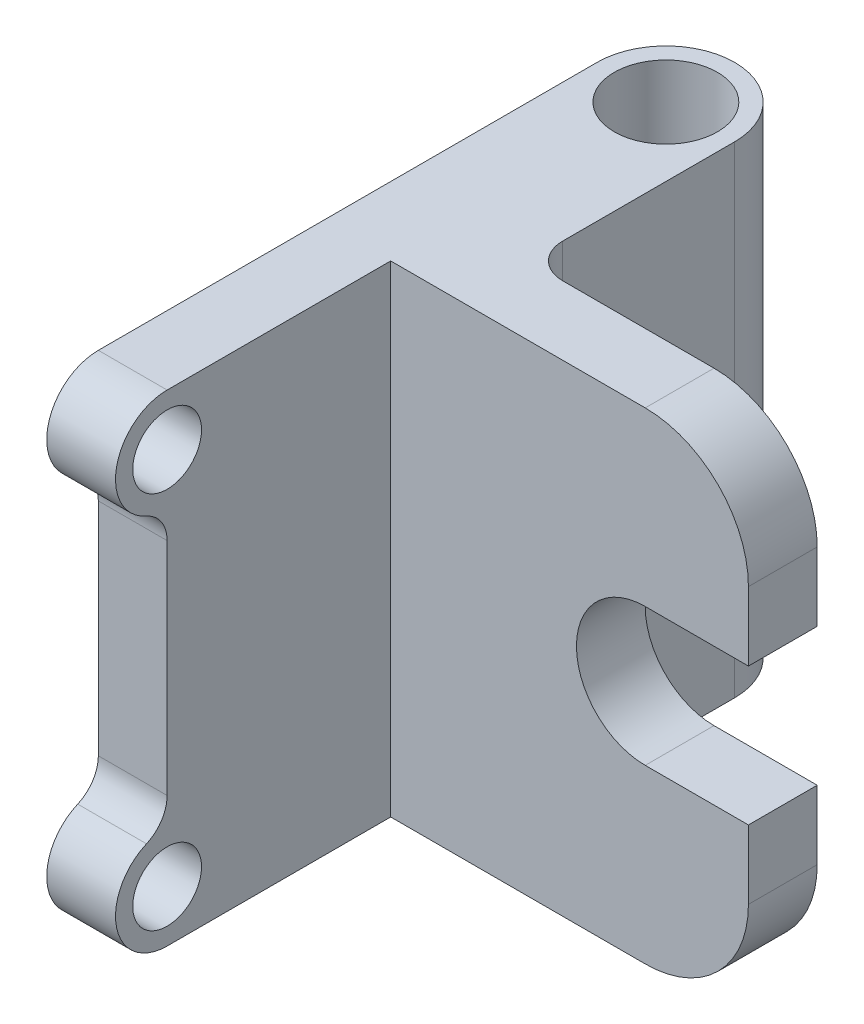
ISO-10303-21;
HEADER;
FILE_DESCRIPTION(('STEP AP214'),'2;1');
FILE_NAME('part.step','',(''),(''),'','','');
FILE_SCHEMA(('AUTOMOTIVE_DESIGN { 1 0 10303 214 1 1 1 1 }'));
ENDSEC;
DATA;
#1=APPLICATION_CONTEXT('core data for automotive mechanical design processes');
#2=APPLICATION_PROTOCOL_DEFINITION('international standard','automotive_design',2000,#1);
#3=PRODUCT_CONTEXT('',#1,'mechanical');
#4=PRODUCT('Part','Part','',(#3));
#5=PRODUCT_RELATED_PRODUCT_CATEGORY('part','',(#4));
#6=PRODUCT_DEFINITION_FORMATION('','',#4);
#7=PRODUCT_DEFINITION_CONTEXT('part definition',#1,'design');
#8=PRODUCT_DEFINITION('design','',#6,#7);
#9=PRODUCT_DEFINITION_SHAPE('','',#8);
#10=(LENGTH_UNIT() NAMED_UNIT(*) SI_UNIT(.MILLI.,.METRE.));
#11=(NAMED_UNIT(*) PLANE_ANGLE_UNIT() SI_UNIT($,.RADIAN.));
#12=(NAMED_UNIT(*) SI_UNIT($,.STERADIAN.) SOLID_ANGLE_UNIT());
#13=UNCERTAINTY_MEASURE_WITH_UNIT(LENGTH_MEASURE(1.E-05),#10,'distance_accuracy_value','');
#14=(GEOMETRIC_REPRESENTATION_CONTEXT(3) GLOBAL_UNCERTAINTY_ASSIGNED_CONTEXT((#13)) GLOBAL_UNIT_ASSIGNED_CONTEXT((#10,
#11,#12)) REPRESENTATION_CONTEXT('',''));
#15=CARTESIAN_POINT('',(0.,0.,0.));
#16=DIRECTION('',(0.,0.,1.));
#17=DIRECTION('',(1.,0.,0.));
#18=AXIS2_PLACEMENT_3D('',#15,#16,#17);
#19=CARTESIAN_POINT('',(47.,15.,0.));
#20=DIRECTION('',(0.,0.,-1.));
#21=DIRECTION('',(-1.,0.,0.));
#22=AXIS2_PLACEMENT_3D('',#19,#20,#21);
#23=PLANE('',#22);
#24=DIRECTION('',(0.,1.,0.));
#25=VECTOR('',#24,1.);
#26=CARTESIAN_POINT('',(25.,0.,0.));
#27=LINE('',#26,#25);
#28=CARTESIAN_POINT('',(25.,0.,0.));
#29=VERTEX_POINT('',#28);
#30=CARTESIAN_POINT('',(25.,70.,0.));
#31=VERTEX_POINT('',#30);
#32=EDGE_CURVE('E69',#29,#31,#27,.T.);
#33=ORIENTED_EDGE('',*,*,#32,.T.);
#34=DIRECTION('',(-1.,0.,0.));
#35=VECTOR('',#34,1.);
#36=CARTESIAN_POINT('',(46.9999999999999,70.,0.));
#37=LINE('',#36,#35);
#38=CARTESIAN_POINT('',(46.9999999999999,70.,0.));
#39=VERTEX_POINT('',#38);
#40=EDGE_CURVE('E270',#39,#31,#37,.T.);
#41=ORIENTED_EDGE('',*,*,#40,.F.);
#42=CARTESIAN_POINT('',(47.,55.,0.));
#43=DIRECTION('',(0.,0.,1.));
#44=DIRECTION('',(1.,0.,0.));
#45=AXIS2_PLACEMENT_3D('',#42,#43,#44);
#46=CIRCLE('',#45,15.);
#47=CARTESIAN_POINT('',(62.,54.9999999999999,0.));
#48=VERTEX_POINT('',#47);
#49=EDGE_CURVE('E296',#48,#39,#46,.T.);
#50=ORIENTED_EDGE('',*,*,#49,.F.);
#51=DIRECTION('',(0.,1.,0.));
#52=VECTOR('',#51,1.);
#53=CARTESIAN_POINT('',(62.,45.,0.));
#54=LINE('',#53,#52);
#55=CARTESIAN_POINT('',(62.,45.,0.));
#56=VERTEX_POINT('',#55);
#57=EDGE_CURVE('E298',#56,#48,#54,.T.);
#58=ORIENTED_EDGE('',*,*,#57,.F.);
#59=DIRECTION('',(1.,0.,0.));
#60=VECTOR('',#59,1.);
#61=CARTESIAN_POINT('',(62.,45.,0.));
#62=LINE('',#61,#60);
#63=CARTESIAN_POINT('',(47.,45.,0.));
#64=VERTEX_POINT('',#63);
#65=EDGE_CURVE('E295',#64,#56,#62,.T.);
#66=ORIENTED_EDGE('',*,*,#65,.F.);
#67=CARTESIAN_POINT('',(47.,35.,0.));
#68=DIRECTION('',(0.,0.,-1.));
#69=DIRECTION('',(1.,0.,0.));
#70=AXIS2_PLACEMENT_3D('',#67,#68,#69);
#71=CIRCLE('',#70,10.);
#72=CARTESIAN_POINT('',(47.,25.,0.));
#73=VERTEX_POINT('',#72);
#74=EDGE_CURVE('E292',#73,#64,#71,.T.);
#75=ORIENTED_EDGE('',*,*,#74,.F.);
#76=DIRECTION('',(-1.,0.,0.));
#77=VECTOR('',#76,1.);
#78=CARTESIAN_POINT('',(47.,25.,0.));
#79=LINE('',#78,#77);
#80=CARTESIAN_POINT('',(62.,25.,0.));
#81=VERTEX_POINT('',#80);
#82=EDGE_CURVE('E287',#81,#73,#79,.T.);
#83=ORIENTED_EDGE('',*,*,#82,.F.);
#84=DIRECTION('',(0.,1.,0.));
#85=VECTOR('',#84,1.);
#86=CARTESIAN_POINT('',(62.,15.0000000000001,0.));
#87=LINE('',#86,#85);
#88=CARTESIAN_POINT('',(62.,15.0000000000001,0.));
#89=VERTEX_POINT('',#88);
#90=EDGE_CURVE('E290',#89,#81,#87,.T.);
#91=ORIENTED_EDGE('',*,*,#90,.F.);
#92=CARTESIAN_POINT('',(47.,15.,0.));
#93=DIRECTION('',(0.,0.,1.));
#94=DIRECTION('',(-1.,0.,0.));
#95=AXIS2_PLACEMENT_3D('',#92,#93,#94);
#96=CIRCLE('',#95,15.);
#97=CARTESIAN_POINT('',(46.9999999999999,0.,0.));
#98=VERTEX_POINT('',#97);
#99=EDGE_CURVE('E289',#98,#89,#96,.T.);
#100=ORIENTED_EDGE('',*,*,#99,.F.);
#101=DIRECTION('',(1.,0.,0.));
#102=VECTOR('',#101,1.);
#103=CARTESIAN_POINT('',(0.,0.,0.));
#104=LINE('',#103,#102);
#105=EDGE_CURVE('E61',#29,#98,#104,.T.);
#106=ORIENTED_EDGE('',*,*,#105,.F.);
#107=EDGE_LOOP('',(#33,#41,#50,#58,#66,#75,#83,#91,#100,#106));
#108=FACE_BOUND('',#107,.T.);
#109=ADVANCED_FACE('F50',(#108),#23,.T.);
#110=CARTESIAN_POINT('',(10.,70.,42.5));
#111=DIRECTION('',(0.,0.,1.));
#112=DIRECTION('',(1.,0.,0.));
#113=AXIS2_PLACEMENT_3D('',#110,#111,#112);
#114=PLANE('',#113);
#115=DIRECTION('',(0.,1.,0.));
#116=VECTOR('',#115,1.);
#117=CARTESIAN_POINT('',(0.,70.,42.5));
#118=LINE('',#117,#116);
#119=CARTESIAN_POINT('',(0.,18.9564392373896,42.5));
#120=VERTEX_POINT('',#119);
#121=CARTESIAN_POINT('',(0.,51.0435607626104,42.5));
#122=VERTEX_POINT('',#121);
#123=EDGE_CURVE('E250',#120,#122,#118,.T.);
#124=ORIENTED_EDGE('',*,*,#123,.F.);
#125=DIRECTION('',(1.,0.,0.));
#126=VECTOR('',#125,1.);
#127=CARTESIAN_POINT('',(0.,18.9564392373896,42.5));
#128=LINE('',#127,#126);
#129=CARTESIAN_POINT('',(10.,18.9564392373896,42.5));
#130=VERTEX_POINT('',#129);
#131=EDGE_CURVE('E230',#120,#130,#128,.T.);
#132=ORIENTED_EDGE('',*,*,#131,.T.);
#133=DIRECTION('',(0.,1.,0.));
#134=VECTOR('',#133,1.);
#135=CARTESIAN_POINT('',(10.,70.,42.5));
#136=LINE('',#135,#134);
#137=CARTESIAN_POINT('',(10.,51.0435607626104,42.5));
#138=VERTEX_POINT('',#137);
#139=EDGE_CURVE('E253',#130,#138,#136,.T.);
#140=ORIENTED_EDGE('',*,*,#139,.T.);
#141=DIRECTION('',(1.,0.,0.));
#142=VECTOR('',#141,1.);
#143=CARTESIAN_POINT('',(0.,51.0435607626104,42.5));
#144=LINE('',#143,#142);
#145=EDGE_CURVE('E239',#122,#138,#144,.T.);
#146=ORIENTED_EDGE('',*,*,#145,.F.);
#147=EDGE_LOOP('',(#124,#132,#140,#146));
#148=FACE_BOUND('',#147,.T.);
#149=ADVANCED_FACE('F360',(#148),#114,.T.);
#150=CARTESIAN_POINT('',(0.,70.,10.));
#151=DIRECTION('',(1.,0.,0.));
#152=DIRECTION('',(0.,0.,-1.));
#153=AXIS2_PLACEMENT_3D('',#150,#151,#152);
#154=PLANE('',#153);
#155=CARTESIAN_POINT('',(0.,62.5,42.5));
#156=DIRECTION('',(1.,0.,0.));
#157=DIRECTION('',(0.,0.,-1.));
#158=AXIS2_PLACEMENT_3D('',#155,#156,#157);
#159=CIRCLE('',#158,5.);
#160=CARTESIAN_POINT('',(0.,62.5,37.5));
#161=VERTEX_POINT('',#160);
#162=EDGE_CURVE('E209',#161,#161,#159,.T.);
#163=ORIENTED_EDGE('',*,*,#162,.T.);
#164=EDGE_LOOP('',(#163));
#165=FACE_BOUND('',#164,.T.);
#166=CARTESIAN_POINT('',(0.,7.5,42.5));
#167=DIRECTION('',(1.,0.,0.));
#168=DIRECTION('',(0.,0.,-1.));
#169=AXIS2_PLACEMENT_3D('',#166,#167,#168);
#170=CIRCLE('',#169,5.);
#171=CARTESIAN_POINT('',(0.,7.5,37.5));
#172=VERTEX_POINT('',#171);
#173=EDGE_CURVE('E205',#172,#172,#170,.T.);
#174=ORIENTED_EDGE('',*,*,#173,.T.);
#175=EDGE_LOOP('',(#174));
#176=FACE_BOUND('',#175,.T.);
#177=DIRECTION('',(0.,0.,-1.));
#178=VECTOR('',#177,1.);
#179=CARTESIAN_POINT('',(0.,70.,10.));
#180=LINE('',#179,#178);
#181=CARTESIAN_POINT('',(0.,70.,42.5));
#182=VERTEX_POINT('',#181);
#183=CARTESIAN_POINT('',(0.,70.,-30.));
#184=VERTEX_POINT('',#183);
#185=EDGE_CURVE('E198',#182,#184,#180,.T.);
#186=ORIENTED_EDGE('',*,*,#185,.T.);
#187=DIRECTION('',(0.,-1.,0.));
#188=VECTOR('',#187,1.);
#189=CARTESIAN_POINT('',(0.,70.,-30.));
#190=LINE('',#189,#188);
#191=CARTESIAN_POINT('',(0.,0.,-30.));
#192=VERTEX_POINT('',#191);
#193=EDGE_CURVE('E177',#184,#192,#190,.T.);
#194=ORIENTED_EDGE('',*,*,#193,.T.);
#195=DIRECTION('',(0.,0.,-1.));
#196=VECTOR('',#195,1.);
#197=CARTESIAN_POINT('',(0.,0.,10.));
#198=LINE('',#197,#196);
#199=CARTESIAN_POINT('',(0.,0.,42.5));
#200=VERTEX_POINT('',#199);
#201=EDGE_CURVE('E11',#200,#192,#198,.T.);
#202=ORIENTED_EDGE('',*,*,#201,.F.);
#203=CARTESIAN_POINT('',(0.,7.5,42.5));
#204=DIRECTION('',(1.,0.,0.));
#205=DIRECTION('',(0.,0.,-1.));
#206=AXIS2_PLACEMENT_3D('',#203,#204,#205);
#207=CIRCLE('',#206,7.50000000000001);
#208=CARTESIAN_POINT('',(0.,14.3738635424338,45.5));
#209=VERTEX_POINT('',#208);
#210=EDGE_CURVE('E224',#209,#200,#207,.T.);
#211=ORIENTED_EDGE('',*,*,#210,.F.);
#212=CARTESIAN_POINT('',(0.,18.9564392373896,47.5));
#213=DIRECTION('',(1.,0.,0.));
#214=DIRECTION('',(0.,0.,-1.));
#215=AXIS2_PLACEMENT_3D('',#212,#213,#214);
#216=CIRCLE('',#215,5.);
#217=EDGE_CURVE('E220',#209,#120,#216,.T.);
#218=ORIENTED_EDGE('',*,*,#217,.T.);
#219=ORIENTED_EDGE('',*,*,#123,.T.);
#220=CARTESIAN_POINT('',(0.,51.0435607626104,47.5));
#221=DIRECTION('',(1.,0.,0.));
#222=DIRECTION('',(0.,0.,-1.));
#223=AXIS2_PLACEMENT_3D('',#220,#221,#222);
#224=CIRCLE('',#223,5.);
#225=CARTESIAN_POINT('',(0.,55.6261364575662,45.5));
#226=VERTEX_POINT('',#225);
#227=EDGE_CURVE('E234',#122,#226,#224,.T.);
#228=ORIENTED_EDGE('',*,*,#227,.T.);
#229=CARTESIAN_POINT('',(0.,62.5,42.5));
#230=DIRECTION('',(1.,0.,0.));
#231=DIRECTION('',(0.,0.,-1.));
#232=AXIS2_PLACEMENT_3D('',#229,#230,#231);
#233=CIRCLE('',#232,7.50000000000001);
#234=EDGE_CURVE('E236',#182,#226,#233,.T.);
#235=ORIENTED_EDGE('',*,*,#234,.F.);
#236=EDGE_LOOP('',(#186,#194,#202,#211,#218,#219,#228,#235));
#237=FACE_BOUND('',#236,.T.);
#238=ADVANCED_FACE('F47',(#165,#176,#237),#154,.F.);
#239=CARTESIAN_POINT('',(0.,0.,10.));
#240=DIRECTION('',(0.,1.,0.));
#241=DIRECTION('',(0.,0.,1.));
#242=AXIS2_PLACEMENT_3D('',#239,#240,#241);
#243=PLANE('',#242);
#244=CARTESIAN_POINT('',(10.,0.,-30.));
#245=DIRECTION('',(0.,1.,0.));
#246=DIRECTION('',(0.,0.,1.));
#247=AXIS2_PLACEMENT_3D('',#244,#245,#246);
#248=CIRCLE('',#247,7.5);
#249=CARTESIAN_POINT('',(10.,0.,-22.5));
#250=VERTEX_POINT('',#249);
#251=EDGE_CURVE('E375',#250,#250,#248,.T.);
#252=ORIENTED_EDGE('',*,*,#251,.T.);
#253=EDGE_LOOP('',(#252));
#254=FACE_BOUND('',#253,.T.);
#255=CARTESIAN_POINT('',(25.,0.,-5.));
#256=DIRECTION('',(0.,-1.,0.));
#257=DIRECTION('',(0.,0.,1.));
#258=AXIS2_PLACEMENT_3D('',#255,#256,#257);
#259=CIRCLE('',#258,5.);
#260=CARTESIAN_POINT('',(20.,0.,-5.));
#261=VERTEX_POINT('',#260);
#262=EDGE_CURVE('E378',#29,#261,#259,.T.);
#263=ORIENTED_EDGE('',*,*,#262,.F.);
#264=ORIENTED_EDGE('',*,*,#105,.T.);
#265=DIRECTION('',(0.,0.,-1.));
#266=VECTOR('',#265,1.);
#267=CARTESIAN_POINT('',(46.9999999999999,0.,10.));
#268=LINE('',#267,#266);
#269=CARTESIAN_POINT('',(46.9999999999999,0.,10.));
#270=VERTEX_POINT('',#269);
#271=EDGE_CURVE('E54',#270,#98,#268,.T.);
#272=ORIENTED_EDGE('',*,*,#271,.F.);
#273=DIRECTION('',(1.,0.,0.));
#274=VECTOR('',#273,1.);
#275=CARTESIAN_POINT('',(0.,0.,10.));
#276=LINE('',#275,#274);
#277=CARTESIAN_POINT('',(10.,0.,10.));
#278=VERTEX_POINT('',#277);
#279=EDGE_CURVE('E262',#278,#270,#276,.T.);
#280=ORIENTED_EDGE('',*,*,#279,.F.);
#281=DIRECTION('',(0.,0.,1.));
#282=VECTOR('',#281,1.);
#283=CARTESIAN_POINT('',(10.,0.,42.5));
#284=LINE('',#283,#282);
#285=CARTESIAN_POINT('',(10.,0.,42.5));
#286=VERTEX_POINT('',#285);
#287=EDGE_CURVE('E254',#278,#286,#284,.T.);
#288=ORIENTED_EDGE('',*,*,#287,.T.);
#289=DIRECTION('',(-1.,0.,0.));
#290=VECTOR('',#289,1.);
#291=CARTESIAN_POINT('',(10.,0.,42.5));
#292=LINE('',#291,#290);
#293=EDGE_CURVE('E195',#286,#200,#292,.T.);
#294=ORIENTED_EDGE('',*,*,#293,.T.);
#295=ORIENTED_EDGE('',*,*,#201,.T.);
#296=CARTESIAN_POINT('',(10.,0.,-30.));
#297=DIRECTION('',(0.,1.,0.));
#298=DIRECTION('',(0.,0.,1.));
#299=AXIS2_PLACEMENT_3D('',#296,#297,#298);
#300=CIRCLE('',#299,10.);
#301=CARTESIAN_POINT('',(20.,0.,-30.));
#302=VERTEX_POINT('',#301);
#303=EDGE_CURVE('E176',#302,#192,#300,.T.);
#304=ORIENTED_EDGE('',*,*,#303,.F.);
#305=DIRECTION('',(0.,0.,1.));
#306=VECTOR('',#305,1.);
#307=CARTESIAN_POINT('',(20.,0.,-30.));
#308=LINE('',#307,#306);
#309=EDGE_CURVE('E202',#302,#261,#308,.T.);
#310=ORIENTED_EDGE('',*,*,#309,.T.);
#311=EDGE_LOOP('',(#263,#264,#272,#280,#288,#294,#295,#304,#310));
#312=FACE_BOUND('',#311,.T.);
#313=ADVANCED_FACE('F194',(#254,#312),#243,.F.);
#314=CARTESIAN_POINT('',(47.,15.,10.));
#315=DIRECTION('',(0.,0.,-1.));
#316=DIRECTION('',(-1.,0.,0.));
#317=AXIS2_PLACEMENT_3D('',#314,#315,#316);
#318=CYLINDRICAL_SURFACE('',#317,15.);
#319=ORIENTED_EDGE('',*,*,#99,.T.);
#320=DIRECTION('',(0.,0.,-1.));
#321=VECTOR('',#320,1.);
#322=CARTESIAN_POINT('',(62.,15.0000000000001,10.));
#323=LINE('',#322,#321);
#324=CARTESIAN_POINT('',(62.,15.0000000000001,10.));
#325=VERTEX_POINT('',#324);
#326=EDGE_CURVE('E318',#325,#89,#323,.T.);
#327=ORIENTED_EDGE('',*,*,#326,.F.);
#328=CARTESIAN_POINT('',(47.,15.,10.));
#329=DIRECTION('',(0.,0.,1.));
#330=DIRECTION('',(-1.,0.,0.));
#331=AXIS2_PLACEMENT_3D('',#328,#329,#330);
#332=CIRCLE('',#331,15.);
#333=EDGE_CURVE('E266',#270,#325,#332,.T.);
#334=ORIENTED_EDGE('',*,*,#333,.F.);
#335=ORIENTED_EDGE('',*,*,#271,.T.);
#336=EDGE_LOOP('',(#319,#327,#334,#335));
#337=FACE_BOUND('',#336,.T.);
#338=ADVANCED_FACE('F329',(#337),#318,.T.);
#339=CARTESIAN_POINT('',(62.,15.0000000000001,10.));
#340=DIRECTION('',(-1.,0.,0.));
#341=DIRECTION('',(0.,0.,1.));
#342=AXIS2_PLACEMENT_3D('',#339,#340,#341);
#343=PLANE('',#342);
#344=ORIENTED_EDGE('',*,*,#90,.T.);
#345=DIRECTION('',(0.,0.,-1.));
#346=VECTOR('',#345,1.);
#347=CARTESIAN_POINT('',(62.,25.,10.));
#348=LINE('',#347,#346);
#349=CARTESIAN_POINT('',(62.,25.,10.));
#350=VERTEX_POINT('',#349);
#351=EDGE_CURVE('E320',#350,#81,#348,.T.);
#352=ORIENTED_EDGE('',*,*,#351,.F.);
#353=DIRECTION('',(0.,1.,0.));
#354=VECTOR('',#353,1.);
#355=CARTESIAN_POINT('',(62.,15.0000000000001,10.));
#356=LINE('',#355,#354);
#357=EDGE_CURVE('E267',#325,#350,#356,.T.);
#358=ORIENTED_EDGE('',*,*,#357,.F.);
#359=ORIENTED_EDGE('',*,*,#326,.T.);
#360=EDGE_LOOP('',(#344,#352,#358,#359));
#361=FACE_BOUND('',#360,.T.);
#362=ADVANCED_FACE('F333',(#361),#343,.F.);
#363=CARTESIAN_POINT('',(47.,25.,10.));
#364=DIRECTION('',(0.,-1.,0.));
#365=DIRECTION('',(0.,0.,-1.));
#366=AXIS2_PLACEMENT_3D('',#363,#364,#365);
#367=PLANE('',#366);
#368=ORIENTED_EDGE('',*,*,#82,.T.);
#369=DIRECTION('',(0.,0.,-1.));
#370=VECTOR('',#369,1.);
#371=CARTESIAN_POINT('',(47.,25.,10.));
#372=LINE('',#371,#370);
#373=CARTESIAN_POINT('',(47.,25.,10.));
#374=VERTEX_POINT('',#373);
#375=EDGE_CURVE('E313',#374,#73,#372,.T.);
#376=ORIENTED_EDGE('',*,*,#375,.F.);
#377=DIRECTION('',(-1.,0.,0.));
#378=VECTOR('',#377,1.);
#379=CARTESIAN_POINT('',(47.,25.,10.));
#380=LINE('',#379,#378);
#381=EDGE_CURVE('E275',#350,#374,#380,.T.);
#382=ORIENTED_EDGE('',*,*,#381,.F.);
#383=ORIENTED_EDGE('',*,*,#351,.T.);
#384=EDGE_LOOP('',(#368,#376,#382,#383));
#385=FACE_BOUND('',#384,.T.);
#386=ADVANCED_FACE('F336',(#385),#367,.F.);
#387=CARTESIAN_POINT('',(47.,35.,10.));
#388=DIRECTION('',(0.,0.,-1.));
#389=DIRECTION('',(-1.,0.,0.));
#390=AXIS2_PLACEMENT_3D('',#387,#388,#389);
#391=CYLINDRICAL_SURFACE('',#390,10.);
#392=ORIENTED_EDGE('',*,*,#74,.T.);
#393=DIRECTION('',(0.,0.,-1.));
#394=VECTOR('',#393,1.);
#395=CARTESIAN_POINT('',(47.,45.,10.));
#396=LINE('',#395,#394);
#397=CARTESIAN_POINT('',(47.,45.,10.));
#398=VERTEX_POINT('',#397);
#399=EDGE_CURVE('E311',#398,#64,#396,.T.);
#400=ORIENTED_EDGE('',*,*,#399,.F.);
#401=CARTESIAN_POINT('',(47.,35.,10.));
#402=DIRECTION('',(0.,0.,-1.));
#403=DIRECTION('',(1.,0.,0.));
#404=AXIS2_PLACEMENT_3D('',#401,#402,#403);
#405=CIRCLE('',#404,10.);
#406=EDGE_CURVE('E274',#374,#398,#405,.T.);
#407=ORIENTED_EDGE('',*,*,#406,.F.);
#408=ORIENTED_EDGE('',*,*,#375,.T.);
#409=EDGE_LOOP('',(#392,#400,#407,#408));
#410=FACE_BOUND('',#409,.T.);
#411=ADVANCED_FACE('F410',(#410),#391,.F.);
#412=CARTESIAN_POINT('',(62.,45.,10.));
#413=DIRECTION('',(0.,1.,0.));
#414=DIRECTION('',(0.,0.,1.));
#415=AXIS2_PLACEMENT_3D('',#412,#413,#414);
#416=PLANE('',#415);
#417=ORIENTED_EDGE('',*,*,#65,.T.);
#418=DIRECTION('',(0.,0.,-1.));
#419=VECTOR('',#418,1.);
#420=CARTESIAN_POINT('',(62.,45.,10.));
#421=LINE('',#420,#419);
#422=CARTESIAN_POINT('',(62.,45.,10.));
#423=VERTEX_POINT('',#422);
#424=EDGE_CURVE('E308',#423,#56,#421,.T.);
#425=ORIENTED_EDGE('',*,*,#424,.F.);
#426=DIRECTION('',(1.,0.,0.));
#427=VECTOR('',#426,1.);
#428=CARTESIAN_POINT('',(62.,45.,10.));
#429=LINE('',#428,#427);
#430=EDGE_CURVE('E279',#398,#423,#429,.T.);
#431=ORIENTED_EDGE('',*,*,#430,.F.);
#432=ORIENTED_EDGE('',*,*,#399,.T.);
#433=EDGE_LOOP('',(#417,#425,#431,#432));
#434=FACE_BOUND('',#433,.T.);
#435=ADVANCED_FACE('F409',(#434),#416,.F.);
#436=CARTESIAN_POINT('',(62.,45.,10.));
#437=DIRECTION('',(-1.,0.,0.));
#438=DIRECTION('',(0.,0.,1.));
#439=AXIS2_PLACEMENT_3D('',#436,#437,#438);
#440=PLANE('',#439);
#441=ORIENTED_EDGE('',*,*,#57,.T.);
#442=DIRECTION('',(0.,0.,-1.));
#443=VECTOR('',#442,1.);
#444=CARTESIAN_POINT('',(62.,54.9999999999999,10.));
#445=LINE('',#444,#443);
#446=CARTESIAN_POINT('',(62.,54.9999999999999,10.));
#447=VERTEX_POINT('',#446);
#448=EDGE_CURVE('E304',#447,#48,#445,.T.);
#449=ORIENTED_EDGE('',*,*,#448,.F.);
#450=DIRECTION('',(0.,1.,0.));
#451=VECTOR('',#450,1.);
#452=CARTESIAN_POINT('',(62.,45.,10.));
#453=LINE('',#452,#451);
#454=EDGE_CURVE('E280',#423,#447,#453,.T.);
#455=ORIENTED_EDGE('',*,*,#454,.F.);
#456=ORIENTED_EDGE('',*,*,#424,.T.);
#457=EDGE_LOOP('',(#441,#449,#455,#456));
#458=FACE_BOUND('',#457,.T.);
#459=ADVANCED_FACE('F405',(#458),#440,.F.);
#460=CARTESIAN_POINT('',(47.,55.,10.));
#461=DIRECTION('',(0.,0.,-1.));
#462=DIRECTION('',(-1.,0.,0.));
#463=AXIS2_PLACEMENT_3D('',#460,#461,#462);
#464=CYLINDRICAL_SURFACE('',#463,15.);
#465=ORIENTED_EDGE('',*,*,#49,.T.);
#466=DIRECTION('',(0.,0.,-1.));
#467=VECTOR('',#466,1.);
#468=CARTESIAN_POINT('',(46.9999999999999,70.,10.));
#469=LINE('',#468,#467);
#470=CARTESIAN_POINT('',(46.9999999999999,70.,10.));
#471=VERTEX_POINT('',#470);
#472=EDGE_CURVE('E305',#471,#39,#469,.T.);
#473=ORIENTED_EDGE('',*,*,#472,.F.);
#474=CARTESIAN_POINT('',(47.,55.,10.));
#475=DIRECTION('',(0.,0.,1.));
#476=DIRECTION('',(1.,0.,0.));
#477=AXIS2_PLACEMENT_3D('',#474,#475,#476);
#478=CIRCLE('',#477,15.);
#479=EDGE_CURVE('E277',#447,#471,#478,.T.);
#480=ORIENTED_EDGE('',*,*,#479,.F.);
#481=ORIENTED_EDGE('',*,*,#448,.T.);
#482=EDGE_LOOP('',(#465,#473,#480,#481));
#483=FACE_BOUND('',#482,.T.);
#484=ADVANCED_FACE('F396',(#483),#464,.T.);
#485=CARTESIAN_POINT('',(46.9999999999999,70.,10.));
#486=DIRECTION('',(0.,-1.,0.));
#487=DIRECTION('',(0.,0.,-1.));
#488=AXIS2_PLACEMENT_3D('',#485,#486,#487);
#489=PLANE('',#488);
#490=CARTESIAN_POINT('',(10.,70.,-30.));
#491=DIRECTION('',(0.,1.,0.));
#492=DIRECTION('',(0.,0.,1.));
#493=AXIS2_PLACEMENT_3D('',#490,#491,#492);
#494=CIRCLE('',#493,7.5);
#495=CARTESIAN_POINT('',(10.,70.,-22.5));
#496=VERTEX_POINT('',#495);
#497=EDGE_CURVE('E374',#496,#496,#494,.T.);
#498=ORIENTED_EDGE('',*,*,#497,.F.);
#499=EDGE_LOOP('',(#498));
#500=FACE_BOUND('',#499,.T.);
#501=ORIENTED_EDGE('',*,*,#40,.T.);
#502=CARTESIAN_POINT('',(25.,70.,-5.));
#503=DIRECTION('',(0.,-1.,0.));
#504=DIRECTION('',(0.,0.,1.));
#505=AXIS2_PLACEMENT_3D('',#502,#503,#504);
#506=CIRCLE('',#505,5.);
#507=CARTESIAN_POINT('',(20.,70.,-5.));
#508=VERTEX_POINT('',#507);
#509=EDGE_CURVE('E187',#31,#508,#506,.T.);
#510=ORIENTED_EDGE('',*,*,#509,.T.);
#511=DIRECTION('',(0.,0.,1.));
#512=VECTOR('',#511,1.);
#513=CARTESIAN_POINT('',(20.,70.,-30.));
#514=LINE('',#513,#512);
#515=CARTESIAN_POINT('',(20.,70.,-30.));
#516=VERTEX_POINT('',#515);
#517=EDGE_CURVE('E371',#516,#508,#514,.T.);
#518=ORIENTED_EDGE('',*,*,#517,.F.);
#519=CARTESIAN_POINT('',(10.,70.,-30.));
#520=DIRECTION('',(0.,1.,0.));
#521=DIRECTION('',(0.,0.,1.));
#522=AXIS2_PLACEMENT_3D('',#519,#520,#521);
#523=CIRCLE('',#522,10.);
#524=EDGE_CURVE('E190',#516,#184,#523,.T.);
#525=ORIENTED_EDGE('',*,*,#524,.T.);
#526=ORIENTED_EDGE('',*,*,#185,.F.);
#527=DIRECTION('',(-1.,0.,0.));
#528=VECTOR('',#527,1.);
#529=CARTESIAN_POINT('',(10.,70.,42.5));
#530=LINE('',#529,#528);
#531=CARTESIAN_POINT('',(10.,70.,42.5));
#532=VERTEX_POINT('',#531);
#533=EDGE_CURVE('E264',#532,#182,#530,.T.);
#534=ORIENTED_EDGE('',*,*,#533,.F.);
#535=DIRECTION('',(0.,0.,-1.));
#536=VECTOR('',#535,1.);
#537=CARTESIAN_POINT('',(10.,70.,10.));
#538=LINE('',#537,#536);
#539=CARTESIAN_POINT('',(10.,70.,10.));
#540=VERTEX_POINT('',#539);
#541=EDGE_CURVE('E256',#532,#540,#538,.T.);
#542=ORIENTED_EDGE('',*,*,#541,.T.);
#543=DIRECTION('',(-1.,0.,0.));
#544=VECTOR('',#543,1.);
#545=CARTESIAN_POINT('',(46.9999999999999,70.,10.));
#546=LINE('',#545,#544);
#547=EDGE_CURVE('E281',#471,#540,#546,.T.);
#548=ORIENTED_EDGE('',*,*,#547,.F.);
#549=ORIENTED_EDGE('',*,*,#472,.T.);
#550=EDGE_LOOP('',(#501,#510,#518,#525,#526,#534,#542,#548,#549));
#551=FACE_BOUND('',#550,.T.);
#552=ADVANCED_FACE('F370',(#500,#551),#489,.F.);
#553=CARTESIAN_POINT('',(47.,15.,10.));
#554=DIRECTION('',(0.,0.,-1.));
#555=DIRECTION('',(-1.,0.,0.));
#556=AXIS2_PLACEMENT_3D('',#553,#554,#555);
#557=PLANE('',#556);
#558=ORIENTED_EDGE('',*,*,#547,.T.);
#559=DIRECTION('',(0.,-1.,0.));
#560=VECTOR('',#559,1.);
#561=CARTESIAN_POINT('',(10.,0.,10.));
#562=LINE('',#561,#560);
#563=EDGE_CURVE('E249',#540,#278,#562,.T.);
#564=ORIENTED_EDGE('',*,*,#563,.T.);
#565=ORIENTED_EDGE('',*,*,#279,.T.);
#566=ORIENTED_EDGE('',*,*,#333,.T.);
#567=ORIENTED_EDGE('',*,*,#357,.T.);
#568=ORIENTED_EDGE('',*,*,#381,.T.);
#569=ORIENTED_EDGE('',*,*,#406,.T.);
#570=ORIENTED_EDGE('',*,*,#430,.T.);
#571=ORIENTED_EDGE('',*,*,#454,.T.);
#572=ORIENTED_EDGE('',*,*,#479,.T.);
#573=EDGE_LOOP('',(#558,#564,#565,#566,#567,#568,#569,#570,#571,#572));
#574=FACE_BOUND('',#573,.T.);
#575=ADVANCED_FACE('F341',(#574),#557,.F.);
#576=CARTESIAN_POINT('',(10.,0.,0.));
#577=DIRECTION('',(1.,0.,0.));
#578=DIRECTION('',(0.,0.,-1.));
#579=AXIS2_PLACEMENT_3D('',#576,#577,#578);
#580=PLANE('',#579);
#581=CARTESIAN_POINT('',(10.,62.5,42.5));
#582=DIRECTION('',(1.,0.,0.));
#583=DIRECTION('',(0.,0.,-1.));
#584=AXIS2_PLACEMENT_3D('',#581,#582,#583);
#585=CIRCLE('',#584,5.);
#586=CARTESIAN_POINT('',(10.,62.5,37.5));
#587=VERTEX_POINT('',#586);
#588=EDGE_CURVE('E215',#587,#587,#585,.T.);
#589=ORIENTED_EDGE('',*,*,#588,.F.);
#590=EDGE_LOOP('',(#589));
#591=FACE_BOUND('',#590,.T.);
#592=CARTESIAN_POINT('',(10.,7.5,42.5));
#593=DIRECTION('',(1.,0.,0.));
#594=DIRECTION('',(0.,0.,-1.));
#595=AXIS2_PLACEMENT_3D('',#592,#593,#594);
#596=CIRCLE('',#595,5.);
#597=CARTESIAN_POINT('',(10.,7.5,37.5));
#598=VERTEX_POINT('',#597);
#599=EDGE_CURVE('E197',#598,#598,#596,.T.);
#600=ORIENTED_EDGE('',*,*,#599,.F.);
#601=EDGE_LOOP('',(#600));
#602=FACE_BOUND('',#601,.T.);
#603=ORIENTED_EDGE('',*,*,#563,.F.);
#604=ORIENTED_EDGE('',*,*,#541,.F.);
#605=CARTESIAN_POINT('',(10.,62.5,42.5));
#606=DIRECTION('',(1.,0.,0.));
#607=DIRECTION('',(0.,0.,-1.));
#608=AXIS2_PLACEMENT_3D('',#605,#606,#607);
#609=CIRCLE('',#608,7.50000000000001);
#610=CARTESIAN_POINT('',(10.,55.6261364575662,45.5));
#611=VERTEX_POINT('',#610);
#612=EDGE_CURVE('E240',#532,#611,#609,.T.);
#613=ORIENTED_EDGE('',*,*,#612,.T.);
#614=CARTESIAN_POINT('',(10.,51.0435607626104,47.5));
#615=DIRECTION('',(1.,0.,0.));
#616=DIRECTION('',(0.,0.,-1.));
#617=AXIS2_PLACEMENT_3D('',#614,#615,#616);
#618=CIRCLE('',#617,5.);
#619=EDGE_CURVE('E235',#138,#611,#618,.T.);
#620=ORIENTED_EDGE('',*,*,#619,.F.);
#621=ORIENTED_EDGE('',*,*,#139,.F.);
#622=CARTESIAN_POINT('',(10.,18.9564392373896,47.5));
#623=DIRECTION('',(1.,0.,0.));
#624=DIRECTION('',(0.,0.,-1.));
#625=AXIS2_PLACEMENT_3D('',#622,#623,#624);
#626=CIRCLE('',#625,5.);
#627=CARTESIAN_POINT('',(10.,14.3738635424338,45.5));
#628=VERTEX_POINT('',#627);
#629=EDGE_CURVE('E211',#628,#130,#626,.T.);
#630=ORIENTED_EDGE('',*,*,#629,.F.);
#631=CARTESIAN_POINT('',(10.,7.5,42.5));
#632=DIRECTION('',(1.,0.,0.));
#633=DIRECTION('',(0.,0.,-1.));
#634=AXIS2_PLACEMENT_3D('',#631,#632,#633);
#635=CIRCLE('',#634,7.50000000000001);
#636=EDGE_CURVE('E221',#628,#286,#635,.T.);
#637=ORIENTED_EDGE('',*,*,#636,.T.);
#638=ORIENTED_EDGE('',*,*,#287,.F.);
#639=EDGE_LOOP('',(#603,#604,#613,#620,#621,#630,#637,#638));
#640=FACE_BOUND('',#639,.T.);
#641=ADVANCED_FACE('F348',(#591,#602,#640),#580,.T.);
#642=CARTESIAN_POINT('',(0.,51.0435607626104,47.5));
#643=DIRECTION('',(1.,0.,0.));
#644=DIRECTION('',(0.,0.,-1.));
#645=AXIS2_PLACEMENT_3D('',#642,#643,#644);
#646=CYLINDRICAL_SURFACE('',#645,5.);
#647=ORIENTED_EDGE('',*,*,#619,.T.);
#648=DIRECTION('',(1.,0.,0.));
#649=VECTOR('',#648,1.);
#650=CARTESIAN_POINT('',(0.,55.6261364575662,45.5));
#651=LINE('',#650,#649);
#652=EDGE_CURVE('E244',#226,#611,#651,.T.);
#653=ORIENTED_EDGE('',*,*,#652,.F.);
#654=ORIENTED_EDGE('',*,*,#227,.F.);
#655=ORIENTED_EDGE('',*,*,#145,.T.);
#656=EDGE_LOOP('',(#647,#653,#654,#655));
#657=FACE_BOUND('',#656,.T.);
#658=ADVANCED_FACE('F363',(#657),#646,.F.);
#659=CARTESIAN_POINT('',(0.,62.5,42.5));
#660=DIRECTION('',(1.,0.,0.));
#661=DIRECTION('',(0.,0.,-1.));
#662=AXIS2_PLACEMENT_3D('',#659,#660,#661);
#663=CYLINDRICAL_SURFACE('',#662,7.50000000000001);
#664=ORIENTED_EDGE('',*,*,#612,.F.);
#665=ORIENTED_EDGE('',*,*,#533,.T.);
#666=ORIENTED_EDGE('',*,*,#234,.T.);
#667=ORIENTED_EDGE('',*,*,#652,.T.);
#668=EDGE_LOOP('',(#664,#665,#666,#667));
#669=FACE_BOUND('',#668,.T.);
#670=ADVANCED_FACE('F364',(#669),#663,.T.);
#671=CARTESIAN_POINT('',(0.,18.9564392373896,47.5));
#672=DIRECTION('',(1.,0.,0.));
#673=DIRECTION('',(0.,0.,-1.));
#674=AXIS2_PLACEMENT_3D('',#671,#672,#673);
#675=CYLINDRICAL_SURFACE('',#674,5.);
#676=ORIENTED_EDGE('',*,*,#629,.T.);
#677=ORIENTED_EDGE('',*,*,#131,.F.);
#678=ORIENTED_EDGE('',*,*,#217,.F.);
#679=DIRECTION('',(1.,0.,0.));
#680=VECTOR('',#679,1.);
#681=CARTESIAN_POINT('',(0.,14.3738635424338,45.5));
#682=LINE('',#681,#680);
#683=EDGE_CURVE('E223',#209,#628,#682,.T.);
#684=ORIENTED_EDGE('',*,*,#683,.T.);
#685=EDGE_LOOP('',(#676,#677,#678,#684));
#686=FACE_BOUND('',#685,.T.);
#687=ADVANCED_FACE('F355',(#686),#675,.F.);
#688=CARTESIAN_POINT('',(0.,7.5,42.5));
#689=DIRECTION('',(1.,0.,0.));
#690=DIRECTION('',(0.,0.,-1.));
#691=AXIS2_PLACEMENT_3D('',#688,#689,#690);
#692=CYLINDRICAL_SURFACE('',#691,7.50000000000001);
#693=ORIENTED_EDGE('',*,*,#636,.F.);
#694=ORIENTED_EDGE('',*,*,#683,.F.);
#695=ORIENTED_EDGE('',*,*,#210,.T.);
#696=ORIENTED_EDGE('',*,*,#293,.F.);
#697=EDGE_LOOP('',(#693,#694,#695,#696));
#698=FACE_BOUND('',#697,.T.);
#699=ADVANCED_FACE('F346',(#698),#692,.T.);
#700=CARTESIAN_POINT('',(0.,7.5,42.5));
#701=DIRECTION('',(1.,0.,0.));
#702=DIRECTION('',(0.,0.,-1.));
#703=AXIS2_PLACEMENT_3D('',#700,#701,#702);
#704=CYLINDRICAL_SURFACE('',#703,5.);
#705=ORIENTED_EDGE('',*,*,#173,.F.);
#706=EDGE_LOOP('',(#705));
#707=FACE_BOUND('',#706,.T.);
#708=ORIENTED_EDGE('',*,*,#599,.T.);
#709=EDGE_LOOP('',(#708));
#710=FACE_BOUND('',#709,.T.);
#711=ADVANCED_FACE('F487',(#707,#710),#704,.F.);
#712=CARTESIAN_POINT('',(0.,62.5,42.5));
#713=DIRECTION('',(1.,0.,0.));
#714=DIRECTION('',(0.,0.,-1.));
#715=AXIS2_PLACEMENT_3D('',#712,#713,#714);
#716=CYLINDRICAL_SURFACE('',#715,5.);
#717=ORIENTED_EDGE('',*,*,#162,.F.);
#718=EDGE_LOOP('',(#717));
#719=FACE_BOUND('',#718,.T.);
#720=ORIENTED_EDGE('',*,*,#588,.T.);
#721=EDGE_LOOP('',(#720));
#722=FACE_BOUND('',#721,.T.);
#723=ADVANCED_FACE('F503',(#719,#722),#716,.F.);
#724=CARTESIAN_POINT('',(20.,0.,-30.));
#725=DIRECTION('',(-1.,0.,0.));
#726=DIRECTION('',(0.,0.,1.));
#727=AXIS2_PLACEMENT_3D('',#724,#725,#726);
#728=PLANE('',#727);
#729=ORIENTED_EDGE('',*,*,#517,.T.);
#730=DIRECTION('',(0.,1.,0.));
#731=VECTOR('',#730,1.);
#732=CARTESIAN_POINT('',(20.,0.,-5.));
#733=LINE('',#732,#731);
#734=EDGE_CURVE('E384',#261,#508,#733,.T.);
#735=ORIENTED_EDGE('',*,*,#734,.F.);
#736=ORIENTED_EDGE('',*,*,#309,.F.);
#737=DIRECTION('',(0.,1.,0.));
#738=VECTOR('',#737,1.);
#739=CARTESIAN_POINT('',(20.,0.,-30.));
#740=LINE('',#739,#738);
#741=EDGE_CURVE('E185',#302,#516,#740,.T.);
#742=ORIENTED_EDGE('',*,*,#741,.T.);
#743=EDGE_LOOP('',(#729,#735,#736,#742));
#744=FACE_BOUND('',#743,.T.);
#745=ADVANCED_FACE('F390',(#744),#728,.F.);
#746=CARTESIAN_POINT('',(25.,0.,-5.));
#747=DIRECTION('',(0.,1.,0.));
#748=DIRECTION('',(0.,0.,1.));
#749=AXIS2_PLACEMENT_3D('',#746,#747,#748);
#750=CYLINDRICAL_SURFACE('',#749,5.);
#751=ORIENTED_EDGE('',*,*,#509,.F.);
#752=ORIENTED_EDGE('',*,*,#32,.F.);
#753=ORIENTED_EDGE('',*,*,#262,.T.);
#754=ORIENTED_EDGE('',*,*,#734,.T.);
#755=EDGE_LOOP('',(#751,#752,#753,#754));
#756=FACE_BOUND('',#755,.T.);
#757=ADVANCED_FACE('F394',(#756),#750,.F.);
#758=CARTESIAN_POINT('',(10.,0.,-30.));
#759=DIRECTION('',(0.,1.,0.));
#760=DIRECTION('',(0.,0.,1.));
#761=AXIS2_PLACEMENT_3D('',#758,#759,#760);
#762=CYLINDRICAL_SURFACE('',#761,10.);
#763=ORIENTED_EDGE('',*,*,#524,.F.);
#764=ORIENTED_EDGE('',*,*,#741,.F.);
#765=ORIENTED_EDGE('',*,*,#303,.T.);
#766=ORIENTED_EDGE('',*,*,#193,.F.);
#767=EDGE_LOOP('',(#763,#764,#765,#766));
#768=FACE_BOUND('',#767,.T.);
#769=ADVANCED_FACE('F180',(#768),#762,.T.);
#770=CARTESIAN_POINT('',(10.,0.,-30.));
#771=DIRECTION('',(0.,1.,0.));
#772=DIRECTION('',(0.,0.,1.));
#773=AXIS2_PLACEMENT_3D('',#770,#771,#772);
#774=CYLINDRICAL_SURFACE('',#773,7.5);
#775=ORIENTED_EDGE('',*,*,#251,.F.);
#776=EDGE_LOOP('',(#775));
#777=FACE_BOUND('',#776,.T.);
#778=ORIENTED_EDGE('',*,*,#497,.T.);
#779=EDGE_LOOP('',(#778));
#780=FACE_BOUND('',#779,.T.);
#781=ADVANCED_FACE('F530',(#777,#780),#774,.F.);
#782=CLOSED_SHELL('',(#109,#149,#238,#313,#338,#362,#386,#411,#435,#459,#484,#552,#575,#641,
#658,#670,#687,#699,#711,#723,#745,#757,#769,#781));
#783=MANIFOLD_SOLID_BREP('B2',#782);
#784=ADVANCED_BREP_SHAPE_REPRESENTATION('',(#18,#783),#14);
#785=SHAPE_DEFINITION_REPRESENTATION(#9,#784);
ENDSEC;
END-ISO-10303-21;
